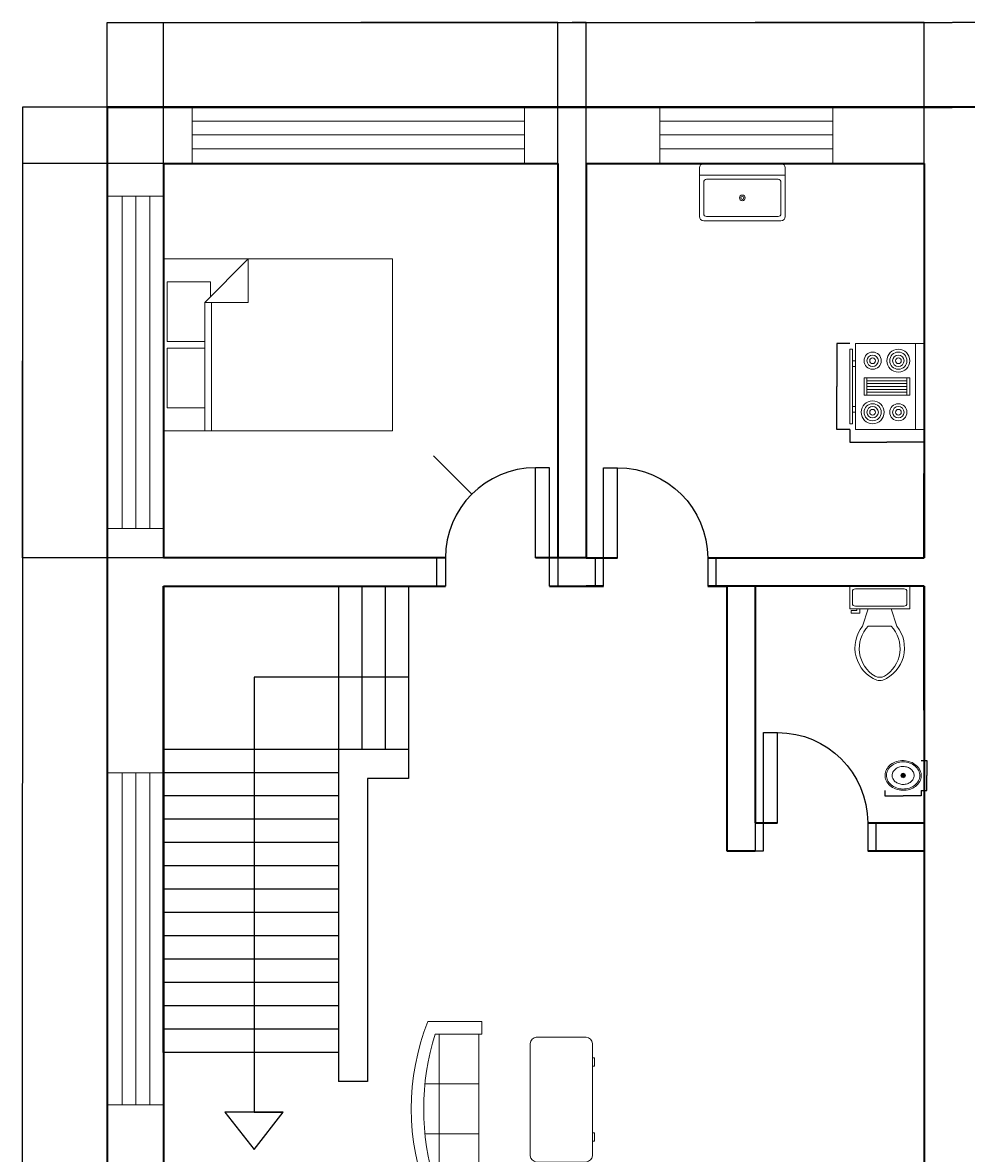
# Model space of a CAD drawing. Units: millimetres. Extents: x 726 to 37095, y -1634 to 13537.
# Tile 1 of 4: x 726 to 9102, y 3500 to 13535. Entities that reach past the tile are written whole.
import ezdxf

# ---------------------------------------------------------------- set-up
doc = ezdxf.new("R2010")
doc.units = ezdxf.units.MM
for name, color, linetype, lineweight in [('A-ANNO-DIMS', 2, 'Continuous', 18), ('A-DOOR', 3, 'Continuous', 25), ('A-EQPM', 8, 'Continuous', 18), ('A-FLOR-FIXT', 9, 'Continuous', 18), ('A-FLOR-STRS', 5, 'Continuous', 25), ('A-FURN', 8, 'Continuous', 18), ('A-GLAZ', 4, 'Continuous', 18), ('A-WALL', 7, 'Continuous', 35)]:
    doc.layers.add(name, color=color, linetype=linetype, lineweight=lineweight)
doc.styles.get("Standard").update_dxf_attribs({"font": 'arial.ttf'})
doc.dimstyles.get("Standard").update_dxf_attribs({"dimtxt": 0.18, "dimasz": 0.18, "dimexe": 0.18, "dimexo": 0.0625, "dimgap": 0.09, "dimtad": 0, "dimtih": 1, "dimtoh": 1, "dimdec": 4, "dimzin": 0, "dimdsep": 46, "dimtxsty": 'Standard', "dimcen": 0.09, "dimadec": 0, "dimazin": 0, "dimtfac": 1, "dimtdec": 4, "dimtofl": 0, "dimtmove": 0, "dimatfit": 3, "dimfxl": 1, "dimtolj": 1, "dimtzin": 0, "dimarcsym": 0})

# ---------------------------------------------------------------- blocks, each defined once
blk = doc.blocks.new('Bed - Queen')
for p, q in [((0, -80.00003000000002), (0, 0)), ((0, 0), (59.99998999999999, 0)), ((59.99998999999999, 0), (59.99998999999999, -80.00003000000002)), ((7.99999, -1.200000000000017), (28.79998, -1.200000000000017)), ((7.99999, -14.4), (7.99999, -1.200000000000017)), ((28.79998, -1.200000000000017), (28.79998, -14.4)), ((31.19999, -1.200000000000017), (51.99999000000001, -1.200000000000017)), ((31.19999, -14.4), (31.19999, -1.200000000000017)), ((51.99999000000001, -1.200000000000017), (51.99999000000001, -16.4)), ((0, -14.4), (44.79999999999999, -14.4)), ((59.99998999999999, -29.60000000000001), (44.79999999999999, -14.4)), ((44.79999999999999, -14.4), (44.79999999999999, -29.60000000000001)), ((44.79999999999999, -16.80000000000001), (0, -16.80000000000001)), ((51.99999000000001, -16.4), (46.79936, -16.4)), ((44.79999999999999, -29.60000000000001), (59.99998999999999, -29.60000000000001)), ((59.99998999999999, -80.00003000000002), (0, -80.00003000000002))]:
    blk.add_line(p, q)
blk = doc.blocks.new('Sofa - Roundback 7 ft.')
for p, q in [((-12.00002, -32.44210000000393), (-12.00003, -6.597100000003898)), ((11.99996999999999, -32.44210000000393), (11.99997999999999, -6.597100000003898)), ((-36.000027, -34.00000000000395), (-36.000027, -11.46960000000396)), ((-35.999844, -13.38190000000397), (35.99979999999999, -13.38190000000397)), ((35.99997999999999, -34.00000000000395), (35.99997999999999, -11.46960000000396)), ((-36.000027, -32.44210000000393), (35.99997999999999, -32.44210000000393))]:
    blk.add_line(p, q)
for points in [[(-36.000027, -34.00000000000395), (-42.000027, -34.00000000000395), (-42.000027, -8.000000000003944)], [(41.99997999999999, -8.000000000003944), (41.99997999999999, -34.00000000000395), (35.99997999999999, -34.00000000000395)]]:
    blk.add_lwpolyline(points)
for centre, radius, start, end in [((0, -114.2500000000039), 114.2500000000039, 68.43141000000072, 111.5686000000006), ((-1.00000000032e-05, -127.1968000000039), 121.1967999999973, 72.72032999999948, 107.2797000000005)]:
    blk.add_arc(centre, radius, start, end)
blk = doc.blocks.new('Desk - 30 x 60 in.')
for p, q in [((-26.999995, 0), (26.999995, 0)), ((-29.999995, -27), (-29.999995, -3)), ((29.999995, -3), (29.999995, -27)), ((26.999995, -30), (-26.999995, -30)), ((-20.000005, -30), (-20.000005, -31)), ((-20.000005, -31), (-16.000005, -31)), ((-16.000005, -31), (-16.000005, -30)), ((15.999995, -31), (15.999995, -30)), ((19.999995, -31), (15.999995, -31)), ((19.999995, -30), (19.999995, -31))]:
    blk.add_line(p, q)
for centre, radius, start, end in [((-26.499995, -3.5), 3.535534000004229, 98.1300999999916, 171.8698999999352), ((26.499995, -3.5), 3.535533999997753, 8.130102000022115, 81.8698999999439), ((-26.499995, -26.5), 3.535534000000845, 188.1301000000653, 261.8699000000085), ((26.499995, -26.5), 3.535534000004826, 278.1301000000561, 351.8698999999439)]:
    blk.add_arc(centre, radius, start, end)
blk = doc.blocks.new('Toilet - top')
for p, q in [((9.5, -6), (9.5, -2)), ((-10, -8.5), (-8, -8.5)), ((-10, -9.5), (-10, -8.5)), ((-7, -9.5), (-10, -9.5)), ((-8, -8.5), (-8, -8)), ((-7, -8), (-7, -9.5)), ((-4, -8), (-6, -14)), ((4, -8), (6, -14)), ((4, -14), (-4, -14))]:
    blk.add_line(p, q)
blk.add_lwpolyline([(10.5, -8), (10.5, 0), (-10.5, 0), (-10.5, -8)], close=True)
for points in [[(-9.5, -2), (-9.5, -6)], [(8.5, -1), (-8.5, -1)], [(-8.5, -7), (8.5, -7)]]:
    blk.add_lwpolyline(points)
for centre, radius, start, end in [((-8.625, -1.875), 0.8838834999999999, 81.86989999999999, 188.1301), ((8.625, -1.875), 0.8838834999999999, 351.8699, 98.13009999999998), ((-8.625, -6.125), 0.8838834999999999, 171.869898, 278.1301), ((8.625, -6.125), 0.8838834999999999, 261.8699, 8.130099999999993), ((3.519562435188956, -21.58049502388982), 12.16902005083646, 141.4691096810948, 247.9714346835576), ((4.199957580658807, -21.81740929088453), 11.3291791325804, 136.3677254423718, 238.946823937405), ((-3.519499936778316, -21.58047137067522), 12.16903423757823, 292.0284332733152, 38.53070636800453), ((-4.199890672038477, -21.81738596564128), 11.32918622148567, 301.0530065773863, 43.63209216694732), ((2.09660981727e-05, -27.87646475467881), 4, 245.7318247449371, 294.2681740488959), ((2.09415214183e-05, -28.99996806116075), 4, 254.8605283244437, 285.1394707718433)]:
    blk.add_arc(centre, radius, start, end)
blk = doc.blocks.new('Sink - Oval top')
for p, q in [((-1, 0), (1, 0)), ((0, 1), (0, -1))]:
    blk.add_line(p, q)
for points in [[(-12.23371880354079, 0.3941914712607968, 0.1176342565883263), (-11.46456229543957, -3.361933235489118, 0.104469279667093), (-8.878748691070427, -6.803541973650567, 0.0900157896014849), (-5.082757700676665, -9.072309807490512, 0.0819199491592185), (-0.3227280122732736, -10.01585280257211, 0.0819199491592091), (4.488169920880977, -9.380701564817912, 0.0900157896014801), (8.422342359155778, -7.36101289847943, 0.1044692796670922), (11.22435122606941, -4.093009071543406, 0.1176342565883338), (12.23371880354091, -0.3941914712607968, 0.1176342565883057), (11.46456229543992, 3.361933235488777, 0.1044692796670849), (8.878748691070427, 6.803541973650567, 0.0900157896014884), (5.082757700676324, 9.072309807490681, 0.0819199491592058), (0.3227280122732736, 10.01585280257211, 0.081919949159207), (-4.488169920880864, 9.380701564817969, 0.0900157896014802), (-8.422342359155778, 7.36101289847943, 0.1044692796670951), (-11.22435122606919, 4.093009071543633, 0.1176342565883402)], [(-11.28627986850119, 0.1590597164737346, 0.1186217001864142), (-10.51590095791209, -3.253161772358112, 0.1046781721811095), (-8.071803350560115, -6.358618019863342, 0.0895620664691738), (-4.537699193222351, -8.366971929609804, 0.0811846988912177), (-0.1289739026695997, -9.15150355811437, 0.0811846988912276), (4.300109150126218, -8.491524865184601, 0.0895620664691798), (7.889406708212618, -6.583562428127606, 0.1046781721811044), (10.42004782883111, -3.548216131892445, 0.1186217001864013), (11.28627986850119, -0.1590597164736209, 0.1186217001863945), (10.51590095791221, 3.253161772357998, 0.1046781721811069), (8.071803350560115, 6.358618019863342, 0.0895620664691756), (4.537699193222124, 8.366971929609917, 0.081184698891216), (0.1289739026695997, 9.151503558114428, 0.0811846988912142), (-4.300109150125877, 8.491524865184829, 0.0895620664691747), (-7.889406708212618, 6.583562428127606, 0.1046781721811045), (-10.42004782883111, 3.548216131892445, 0.1186217001863946)], [(-7.420452389032902, 0.0829876781601797, 0.1182825673856775), (-6.907065465214486, -2.1674649380775, 0.1046074595377274), (-5.294791470712084, -4.209988192029413, 0.0897179636260996), (-2.966599981142508, -5.528122152688069, 0.0814360825277113), (-0.0675135187855176, -6.036810076758797, 0.0814360825277218), (2.84222437824053, -5.593085960977873, 0.0897179636261315), (5.199312936802016, -4.327350491993342, 0.1046074595376878), (6.85686365682659, -2.321395784920355, 0.1182825673856714), (7.420452389033016, -0.0829876781601797, 0.1182825673856961), (6.907065465214486, 2.167464938077614, 0.1046074595377135), (5.294791470712084, 4.209988192029413, 0.0897179636261265), (2.966599981142621, 5.528122152687842, 0.0814360825277426), (0.0675135187855176, 6.036810076758797, 0.0814360825277225), (-2.842224378240644, 5.593085960977873, 0.0897179636261212), (-5.199312936802016, 4.327350491993342, 0.1046074595377049), (-6.856863656826476, 2.321395784920355, 0.1182825673856712)]]:
    blk.add_lwpolyline(points, format="xyb", close=True)
for radius in [1.5, 1]:
    blk.add_circle((0, 0), radius)
blk = doc.blocks.new('Range-Oven - 30 in top')
for p, q in [((0, -3), (30, -3)), ((12, -6), (18, -6)), ((13, -19.999996), (13, -6)), ((14, -6), (14, -19.999996)), ((15, -19.999996), (15, -6)), ((16, -6), (16, -19.999996)), ((17, -19.999996), (17, -6)), ((18, -19.999996), (12, -19.999996)), ((6.000000000000003, -23.99999600000001), (6.000000000000003, -24.999996)), ((8.000000000000004, -24.999996), (8.000000000000004, -23.99999600000001)), ((22.00000000000001, -24.999996), (22.00000000000001, -23.99999600000001)), ((24, -23.99999600000001), (24, -24.999996))]:
    blk.add_line(p, q)
for points in [[(0, -23.99999600000001), (0, 0), (30, 0), (30, -23.99999600000001)], [(12, -20.999996), (12, -5), (18, -5), (18, -20.999996)], [(2.000000000000003, -25.999996), (2.000000000000003, -24.999996), (28.00000000000001, -24.999996), (28.00000000000001, -25.999996)]]:
    blk.add_lwpolyline(points, close=True)
for centre, radius in [((6.000000000000003, -9.0000002), 4), ((6.000000000000003, -9.0000002), 3), ((6.000000000000003, -9.0000002), 2), ((24, -9.0000002), 3), ((24, -9.0000002), 2), ((6.000000000000003, -9.0000002), 1), ((24, -9.0000002), 1), ((6.000000000000003, -18), 3), ((24, -18), 4), ((24, -18), 3), ((6.000000000000003, -18), 2), ((6.000000000000003, -18), 1), ((24, -18), 2), ((24, -18), 1)]:
    blk.add_circle(centre, radius)
blk = doc.blocks.new('Sink-single - 30 in top')
blk.add_line((-15, -3.999996000000001), (15, -3.999996000000001))
for points in [[(-13.5, 0), (13.5, 0)], [(-15, -18.499996), (-15, -1.500000000000001)], [(15, -1.500000000000001), (15, -18.499996)], [(-13.5, -17.499996), (-13.5, -6.499996000000001)], [(-12.5, -5.499996000000001), (12.5, -5.499996000000001)], [(13.5, -6.499996000000001), (13.5, -17.499996)], [(12.5, -18.499996), (-12.5, -18.499996)], [(13.5, -19.999996), (-13.5, -19.999996)]]:
    blk.add_lwpolyline(points)
for radius in [1, 0.5]:
    blk.add_circle((0, -11.999996), radius)
for centre, radius, start, end in [((-13.5, -1.500000000000001), 1.5, 90, 180), ((13.5, -1.500000000000001), 1.5, 0, 90), ((-12.5, -6.499996000000001), 1, 90, 180), ((12.5, -6.499996000000001), 1, 0, 90), ((-13.5, -18.499996), 1.5, 180, 270), ((-12.5, -17.499996), 1, 180, 270), ((12.5, -17.499996), 1, 270, 0), ((13.5, -18.499996), 1.5, 270, 0)]:
    blk.add_arc(centre, radius, start, end)
blk = doc.blocks.new('Window - Wood Frame 36 in. Wide plan')
for p, q in [((0, 6), (0, 0)), ((36, 6), (36, 0)), ((0, 4.5), (36, 4.5)), ((0, 3), (36, 3)), ((0, 1.5), (36, 1.5))]:
    blk.add_line(p, q)
blk = doc.blocks.new('DOOR-SWING-800')
for p, q in [((999.1999999999979, 1050), (874.1999999999979, 1050)), ((874.1999999999979, 250), (874.1999999999979, 1050)), ((999.1999999999979, 250), (999.1999999999979, 1050)), ((9.095e-13, 250), (74.199999999998, 250)), ((9.095e-13, 0), (9.095e-13, 250)), ((74.199999999998, 250), (74.199999999998, 0)), ((874.1999999999979, 250), (999.1999999999979, 250)), ((999.1999999999979, 250), (1073.400000000002, 250)), ((999.1999999999979, 0), (999.1999999999979, 250)), ((1073.400000000002, 250), (1073.400000000002, 0)), ((74.199999999998, 0), (9.095e-13, 0)), ((1073.400000000002, 0), (999.1999999999979, 0))]:
    blk.add_line(p, q)
blk.add_arc((874.1999999999979, 250), 800, 90, 180)
blk = doc.blocks.new('STAIR-QUARTER-TURN')
for p, q in [((1551.94660387568, 5000.000000000002), (1551.94660387568, 3551.516503049365)), ((1758.872817725773, 5000.000000000002), (1758.872817725773, 3551.516503049365)), ((1965.799031575862, 5000.000000000002), (1965.799031575862, 3551.516503049365)), ((2172.725245425954, 5000.000000000002), (2172.725245425954, 3551.516503049365)), ((2172.725245425954, 4193.579423830473), (803.743340616409, 4193.579423830471)), ((803.743340616409, 4193.579423830471), (803.743340616409, 330.5564002077117)), ((2172.725245425954, 3551.516503049366), (0, 3551.516503049365)), ((1551.94660387568, 3551.516503049365), (1551.94660387568, 3344.590289199272)), ((2172.725245425954, 3551.516503049365), (2172.725245425954, 3292.858735736751)), ((1551.94660387568, 3344.590289199272), (0, 3344.590289199273)), ((1551.94660387568, 3344.590289199272), (1551.94660387568, 861.4757229981805)), ((2172.725245425954, 3292.858735736751), (1810.604371188295, 3292.858735736751)), ((1810.604371188295, 3292.85873573675), (1810.604371188295, 602.8179556856148)), ((1551.94660387568, 3137.664075349182), (0, 3137.664075349182)), ((1551.94660387568, 2930.73786149909), (0, 2930.737861499091)), ((1551.94660387568, 2723.811647649), (0, 2723.811647649001)), ((1551.94660387568, 2516.885433798908), (0, 2516.885433798909)), ((1551.94660387568, 2309.959219948817), (0, 2309.959219948818)), ((1551.94660387568, 2103.033006098726), (0, 2103.033006098727)), ((1551.94660387568, 1896.106792248635), (0, 1896.106792248635)), ((1551.94660387568, 1689.180578398543), (0, 1689.180578398544)), ((1551.94660387568, 1482.254364548453), (0, 1482.254364548454)), ((1551.94660387568, 1275.328150698362), (0, 1275.328150698363)), ((1551.94660387568, 1068.40193684827), (0, 1068.401936848271)), ((1551.94660387568, 861.4757229981795), (0, 861.4757229981805)), ((1551.94660387568, 861.4757229981805), (1551.946603875687, 602.8179556856074)), ((1810.604371188295, 602.8179556856148), (1551.946603875687, 602.8179556855675)), ((803.743340616409, 330.5564002077117), (545.0855733037969, 330.5564002077117)), ((545.0855733037969, 330.5564002077117), (803.743340616409, 4.547e-13)), ((803.743340616409, 330.5564002077117), (1062.401107929021, 330.5564002077108)), ((803.743340616409, 4.547e-13), (1062.401107929021, 330.5564002077117))]:
    blk.add_line(p, q)
blk = doc.blocks.new('WIN-1535')
for p, q in [((0, 1.819e-12), (0, 500.0000000000036)), ((1534.861597237876, 1.819e-12), (1534.861597237876, 500.0000000000036)), ((-9.095e-13, 377.1532172399693), (1534.861597237876, 377.1532172399693)), ((-9.095e-13, 254.306434479935), (1534.861597237876, 254.306434479935)), ((-9.095e-13, 131.459651719897), (1534.861597237876, 131.4596517198988))]:
    blk.add_line(p, q)
blk = doc.blocks.new('*D33')
at = {"layer": 'A-ANNO-DIMS', "color": 0, "lineweight": -2, "transparency": 16777216}
for p, q in [((8379.49967440098, 6721.430037603937), (8379.49967440098, 6672.895314363273)), ((8379.67967440098, 6673.075314363273), (8539.884149777998, 6673.075314363273)), ((8702.10116267207, 6673.075314363273), (8541.896687295051, 6673.075314363273)), ((8702.28116267207, 6721.430037603937), (8702.28116267207, 6672.895314363273))]:
    blk.add_line(p, q, dxfattribs=at)
at = {"layer": 'A-ANNO-DIMS', "color": 0, "transparency": 16777216}
for points in [[(8379.67967440098, 6673.105314363273), (8379.67967440098, 6673.045314363275), (8379.49967440098, 6673.075314363273)], [(8702.10116267207, 6673.105314363273), (8702.10116267207, 6673.045314363275), (8702.28116267207, 6673.075314363273)]]:
    blk.add_solid(points, dxfattribs=at)
at = {"layer": 'Defpoints', "color": 0, "transparency": 16777216}
for p in [(8379.49967440098, 6721.492537603937), (8702.28116267207, 6721.492537603937), (8702.28116267207, 6673.075314363273)]:
    blk.add_point(p, dxfattribs=at)
at = {"layer": 'A-ANNO-DIMS', "color": 0, "transparency": 16777216, "insert": (8540.890418536525, 6673.075314363273), "char_height": 0.18, "attachment_point": 5}
blk.add_mtext('\\A1;BASIN 323 TYP.', dxfattribs=at)
blk = doc.blocks.new('*D34')
at = {"layer": 'A-ANNO-DIMS', "color": 0, "lineweight": -2, "transparency": 16777216}
for p, q in [((8702.343662672074, 6986.237226650004), (8750.878385912742, 6986.237226650004)), ((8750.698385912741, 6986.057226650004), (8750.698385912741, 6854.046785264762)), ((8750.698385912741, 6721.672537603942), (8750.698385912741, 6853.682978989183)), ((8702.343662672074, 6721.492537603942), (8750.878385912742, 6721.492537603942))]:
    blk.add_line(p, q, dxfattribs=at)
at = {"layer": 'A-ANNO-DIMS', "color": 0, "transparency": 16777216}
for points in [[(8750.66838591274, 6986.057226650004), (8750.728385912742, 6986.057226650004), (8750.698385912741, 6986.237226650004)], [(8750.66838591274, 6721.672537603942), (8750.728385912742, 6721.672537603942), (8750.698385912741, 6721.492537603942)]]:
    blk.add_solid(points, dxfattribs=at)
at = {"layer": 'Defpoints', "color": 0, "transparency": 16777216}
for p in [(8702.281162672074, 6986.237226650004), (8750.698385912741, 6986.237226650004), (8702.281162672074, 6721.492537603942)]:
    blk.add_point(p, dxfattribs=at)
at = {"layer": 'A-ANNO-DIMS', "color": 0, "transparency": 16777216, "insert": (8750.698385912741, 6853.864882126969), "char_height": 0.18, "attachment_point": 5}
blk.add_mtext('\\A1;265 TYP.', dxfattribs=at)
blk = doc.blocks.new('*D37')
at = {"layer": 'A-ANNO-DIMS', "color": 0, "lineweight": -2, "transparency": 16777216}
for p, q in [((8066.847447465294, 10686.62375609469), (7952.429947465296, 10686.62375609469)), ((7952.609947465297, 10686.44375609469), (7952.609947465297, 10305.80682567177)), ((7952.609947465298, 9924.803756094694), (7952.609947465297, 10305.44068651761)), ((8066.847447465294, 9924.623756094694), (7952.429947465297, 9924.623756094694))]:
    blk.add_line(p, q, dxfattribs=at)
at = {"layer": 'A-ANNO-DIMS', "color": 0, "transparency": 16777216}
for points in [[(7952.579947465297, 10686.44375609469), (7952.639947465296, 10686.44375609469), (7952.609947465297, 10686.62375609469)], [(7952.579947465299, 9924.803756094694), (7952.639947465297, 9924.803756094694), (7952.609947465298, 9924.623756094694)]]:
    blk.add_solid(points, dxfattribs=at)
at = {"layer": 'Defpoints', "color": 0, "transparency": 16777216}
for p in [(8066.909947465294, 10686.62375609469), (7952.609947465298, 9924.623756094694), (8066.909947465294, 9924.623756094694)]:
    blk.add_point(p, dxfattribs=at)
at = {"layer": 'A-ANNO-DIMS', "color": 0, "transparency": 16777216, "insert": (7952.609947465298, 10305.62375609469), "char_height": 0.18, "attachment_point": 5}
blk.add_mtext('\\A1;RANGE 762 TYP.', dxfattribs=at)
blk = doc.blocks.new('*D38')
at = {"layer": 'A-ANNO-DIMS', "color": 0, "lineweight": -2, "transparency": 16777216}
for p, q in [((8066.909947465289, 9924.56125609469), (8066.909947465289, 9810.14375609469)), ((8727.30984586529, 9924.56125609469), (8727.30984586529, 9810.14375609469)), ((8067.089947465289, 9810.32375609469), (8396.511390526133, 9810.32375609469)), ((8727.12984586529, 9810.32375609469), (8397.708402804445, 9810.32375609469))]:
    blk.add_line(p, q, dxfattribs=at)
at = {"layer": 'A-ANNO-DIMS', "color": 0, "transparency": 16777216}
for points in [[(8067.089947465289, 9810.353756094692), (8067.089947465289, 9810.29375609469), (8066.909947465289, 9810.32375609469)], [(8727.12984586529, 9810.353756094692), (8727.12984586529, 9810.29375609469), (8727.30984586529, 9810.32375609469)]]:
    blk.add_solid(points, dxfattribs=at)
at = {"layer": 'Defpoints', "color": 0, "transparency": 16777216}
for p in [(8066.909947465289, 9924.62375609469), (8727.30984586529, 9924.62375609469), (8727.30984586529, 9810.32375609469)]:
    blk.add_point(p, dxfattribs=at)
at = {"layer": 'A-ANNO-DIMS', "color": 0, "transparency": 16777216, "insert": (8397.10989666529, 9810.32375609469), "char_height": 0.18, "attachment_point": 5}
blk.add_mtext('\\A1;660 TYP.', dxfattribs=at)
blk = doc.blocks.new('*D43')
at = {"layer": 'A-ANNO-DIMS', "color": 0, "lineweight": -2, "transparency": 16777216}
for p, q in [((1477.309846, 12783.948368), (1477.309846, 13534.815868)), ((1477.489846, 13534.635868), (8976.889927855387, 13534.635868)), ((16477.129846, 13534.635868), (8977.72976414461, 13534.635868)), ((16477.309846, 12783.948368), (16477.309846, 13534.815868))]:
    blk.add_line(p, q, dxfattribs=at)
at = {"layer": 'A-ANNO-DIMS', "color": 0, "transparency": 16777216}
for points in [[(1477.489846, 13534.665868), (1477.489846, 13534.605868), (1477.309846, 13534.635868)], [(16477.129846, 13534.665868), (16477.129846, 13534.605868), (16477.309846, 13534.635868)]]:
    blk.add_solid(points, dxfattribs=at)
at = {"layer": 'Defpoints', "color": 0, "transparency": 16777216}
for p in [(16477.309846, 13534.635868), (1477.309846, 12783.885868), (16477.309846, 12783.885868)]:
    blk.add_point(p, dxfattribs=at)
at = {"layer": 'A-ANNO-DIMS', "color": 0, "transparency": 16777216, "insert": (8977.309846, 13534.635868), "char_height": 0.18, "attachment_point": 5}
blk.add_mtext('\\A1;15000', dxfattribs=at)
blk = doc.blocks.new('*D44')
at = {"layer": 'A-ANNO-DIMS', "color": 0, "lineweight": -2, "transparency": 16777216}
for p, q in [((1477.247346, 12783.885868), (726.3798459999991, 12783.885868)), ((726.559845999999, 12783.705868), (726.5598460000004, 6784.067771137793)), ((726.5598460000017, 784.0658680000001), (726.5598460000004, 6783.703964862214)), ((1477.247346, 783.8858680000003), (726.3798460000017, 783.8858680000002))]:
    blk.add_line(p, q, dxfattribs=at)
at = {"layer": 'A-ANNO-DIMS', "color": 0, "transparency": 16777216}
for points in [[(726.5298459999991, 12783.705868), (726.589845999999, 12783.705868), (726.559845999999, 12783.885868)], [(726.5298460000017, 784.0658680000001), (726.5898460000016, 784.0658680000001), (726.5598460000017, 783.8858680000002)]]:
    blk.add_solid(points, dxfattribs=at)
at = {"layer": 'Defpoints', "color": 0, "transparency": 16777216}
for p in [(726.559845999999, 12783.885868), (1477.309846, 12783.885868), (1477.309846, 783.8858680000003)]:
    blk.add_point(p, dxfattribs=at)
at = {"layer": 'A-ANNO-DIMS', "color": 0, "transparency": 16777216, "insert": (726.5598460000022, 6783.885868000002), "char_height": 0.18, "attachment_point": 5}
blk.add_mtext('\\A1;12000', dxfattribs=at)
blk = doc.blocks.new('*D45')
at = {"layer": 'A-ANNO-DIMS', "color": 0, "lineweight": -2, "transparency": 16777216}
for p, q in [((1977.309846, 12283.948368), (1977.309846, 13534.815868)), ((1977.489846, 13534.635868), (3726.951442180082, 13534.635868)), ((5477.129846, 13534.635868), (3727.668249819919, 13534.635868)), ((5477.309846, 12283.948368), (5477.309846, 13534.815868))]:
    blk.add_line(p, q, dxfattribs=at)
at = {"layer": 'A-ANNO-DIMS', "color": 0, "transparency": 16777216}
for points in [[(1977.489846, 13534.665868), (1977.489846, 13534.605868), (1977.309846, 13534.635868)], [(5477.129846, 13534.665868), (5477.129846, 13534.605868), (5477.309846, 13534.635868)]]:
    blk.add_solid(points, dxfattribs=at)
at = {"layer": 'Defpoints', "color": 0, "transparency": 16777216}
for p in [(5477.309846, 13534.635868), (1977.309846, 12283.885868), (5477.309846, 12283.885868)]:
    blk.add_point(p, dxfattribs=at)
at = {"layer": 'A-ANNO-DIMS', "color": 0, "transparency": 16777216, "insert": (3727.309846, 13534.635868), "char_height": 0.18, "attachment_point": 5}
blk.add_mtext('\\A1;3500', dxfattribs=at)
blk = doc.blocks.new('*D46')
at = {"layer": 'A-ANNO-DIMS', "color": 0, "lineweight": -2, "transparency": 16777216}
for p, q in [((5477.309846, 12283.948368), (5477.309846, 13534.815868)), ((5477.489846, 13534.635868), (5602.019770965893, 13534.635868)), ((5727.129846, 13534.635868), (5602.599921034107, 13534.635868)), ((5727.309846, 12283.948368), (5727.309846, 13534.815868))]:
    blk.add_line(p, q, dxfattribs=at)
at = {"layer": 'A-ANNO-DIMS', "color": 0, "transparency": 16777216}
for points in [[(5477.489846, 13534.665868), (5477.489846, 13534.605868), (5477.309846, 13534.635868)], [(5727.129846, 13534.665868), (5727.129846, 13534.605868), (5727.309846, 13534.635868)]]:
    blk.add_solid(points, dxfattribs=at)
at = {"layer": 'Defpoints', "color": 0, "transparency": 16777216}
for p in [(5727.309846, 13534.635868), (5477.309846, 12283.885868), (5727.309846, 12283.885868)]:
    blk.add_point(p, dxfattribs=at)
at = {"layer": 'A-ANNO-DIMS', "color": 0, "transparency": 16777216, "insert": (5602.309846, 13534.635868), "char_height": 0.18, "attachment_point": 5}
blk.add_mtext('\\A1;250', dxfattribs=at)
blk = doc.blocks.new('*D47')
at = {"layer": 'A-ANNO-DIMS', "color": 0, "lineweight": -2, "transparency": 16777216}
for p, q in [((5727.309846, 12283.948368), (5727.309846, 13534.815868)), ((5727.489846, 13534.635868), (7226.951442180082, 13534.635868)), ((8727.129846, 13534.635868), (7227.668249819918, 13534.635868)), ((8727.309846, 12283.948368), (8727.309846, 13534.815868))]:
    blk.add_line(p, q, dxfattribs=at)
at = {"layer": 'A-ANNO-DIMS', "color": 0, "transparency": 16777216}
for points in [[(5727.489846, 13534.665868), (5727.489846, 13534.605868), (5727.309846, 13534.635868)], [(8727.129846, 13534.665868), (8727.129846, 13534.605868), (8727.309846, 13534.635868)]]:
    blk.add_solid(points, dxfattribs=at)
at = {"layer": 'Defpoints', "color": 0, "transparency": 16777216}
for p in [(8727.309846, 13534.635868), (5727.309846, 12283.885868), (8727.309846, 12283.885868)]:
    blk.add_point(p, dxfattribs=at)
at = {"layer": 'A-ANNO-DIMS', "color": 0, "transparency": 16777216, "insert": (7227.309846, 13534.635868), "char_height": 0.18, "attachment_point": 5}
blk.add_mtext('\\A1;3000', dxfattribs=at)
blk = doc.blocks.new('*D48')
at = {"layer": 'A-ANNO-DIMS', "color": 0, "lineweight": -2, "transparency": 16777216}
for p, q in [((8727.309846, 12283.948368), (8727.309846, 13534.815868)), ((8727.489846, 13534.635868), (8977.021305754433, 13534.635868)), ((9227.129846, 13534.635868), (8977.598386245567, 13534.635868)), ((9227.309846, 12283.948368), (9227.309846, 13534.815868))]:
    blk.add_line(p, q, dxfattribs=at)
at = {"layer": 'A-ANNO-DIMS', "color": 0, "transparency": 16777216}
for points in [[(8727.489846, 13534.665868), (8727.489846, 13534.605868), (8727.309846, 13534.635868)], [(9227.129846, 13534.665868), (9227.129846, 13534.605868), (9227.309846, 13534.635868)]]:
    blk.add_solid(points, dxfattribs=at)
at = {"layer": 'Defpoints', "color": 0, "transparency": 16777216}
for p in [(9227.309846, 13534.635868), (8727.309846, 12283.885868), (9227.309846, 12283.885868)]:
    blk.add_point(p, dxfattribs=at)
at = {"layer": 'A-ANNO-DIMS', "color": 0, "transparency": 16777216, "insert": (8977.309846, 13534.635868), "char_height": 0.18, "attachment_point": 5}
blk.add_mtext('\\A1;500', dxfattribs=at)
blk = doc.blocks.new('*D53')
at = {"layer": 'A-ANNO-DIMS', "color": 0, "lineweight": -2, "transparency": 16777216}
for p, q in [((1977.247346000001, 12283.885868), (726.3798460000002, 12283.885868)), ((726.5598460000001, 12283.705868), (726.5598460000004, 10534.06783252933)), ((726.5598460000009, 8784.065868000003), (726.5598460000004, 10533.70390347067)), ((1977.247346000001, 8783.885868000005), (726.3798460000007, 8783.885868000005))]:
    blk.add_line(p, q, dxfattribs=at)
at = {"layer": 'A-ANNO-DIMS', "color": 0, "transparency": 16777216}
for points in [[(726.5298460000001, 12283.705868), (726.589846, 12283.705868), (726.5598460000001, 12283.885868)], [(726.5298460000009, 8784.065868000003), (726.5898460000008, 8784.065868000003), (726.5598460000009, 8783.885868000005)]]:
    blk.add_solid(points, dxfattribs=at)
at = {"layer": 'Defpoints', "color": 0, "transparency": 16777216}
for p in [(1977.309846000001, 12283.885868), (726.5598460000009, 8783.885868000005), (1977.309846000001, 8783.885868000005)]:
    blk.add_point(p, dxfattribs=at)
at = {"layer": 'A-ANNO-DIMS', "color": 0, "transparency": 16777216, "insert": (726.5598460000034, 10533.885868), "char_height": 0.18, "attachment_point": 5}
blk.add_mtext('\\A1;3500', dxfattribs=at)
blk = doc.blocks.new('*D85')
at = {"layer": 'A-ANNO-DIMS', "color": 0, "lineweight": -2, "transparency": 16777216}
for p, q in [((4372.832594830522, 9688.981976769475), (4373.012594830522, 9688.981976769475)), ((4373.012594830522, 9688.981976769475), (4712.29678469906, 9349.69821514029)), ((5278.019845999999, 8783.885867999996), (5278.199846, 8783.885868)), ((5278.109846, 8783.795868), (5278.109846, 8783.975868))]:
    blk.add_line(p, q, dxfattribs=at)
at = {"layer": 'A-ANNO-DIMS', "color": 0, "transparency": 16777216}
blk.add_solid([(4712.317997889108, 9349.719428357112), (4712.275571509011, 9349.677001923465), (4712.424063999999, 9349.570936)], dxfattribs=at)
at = {"layer": 'Defpoints', "color": 0, "transparency": 16777216}
for p in [(4712.424063999999, 9349.570936), (5278.109845999999, 8783.885868)]:
    blk.add_point(p, dxfattribs=at)
at = {"layer": 'A-ANNO-DIMS', "color": 0, "transparency": 16777216, "insert": (4372.264047763674, 9688.981976769477), "char_height": 0.18, "attachment_point": 5}
blk.add_mtext('\\A1;6X R800', dxfattribs=at)

msp = doc.modelspace()

# ---------------------------------------------------------------- linework, layer by layer
at = {"layer": 'A-DOOR'}
for p, q in [((5403.109845865284, 8783.885868122885), (5278.109845865284, 8783.885868122885)), ((5807.038045798428, 8783.885868122887), (5807.038045798428, 8533.885868122887)), ((5881.238045798433, 8783.885868122887), (6006.238045798433, 8783.885868122887)), ((7227.309845865285, 6434.561644066505), (7227.309845865285, 6184.561644066505)), ((7301.50984586529, 6434.561644066505), (7426.50984586529, 6434.561644066505)), ((7227.309845865287, 6184.561644066505), (7301.50984586529, 6184.561644066505))]:
    msp.add_line(p, q, dxfattribs=at)
at = {"layer": 'A-FLOR-STRS'}
for p, q in [((2781.053186481699, 7727.465291953355), (2781.053186481699, 7727.465291953355)), ((3039.710953794312, 3864.442268330595), (2781.053186481699, 3864.442268330595))]:
    msp.add_line(p, q, dxfattribs=at)
at = {"layer": 'A-WALL'}
for p, q in [((16477.30984586529, 12783.88586812288), (1477.309845865288, 12783.88586812288)), ((1477.309845865288, 12783.88586812288), (1477.309845865288, 783.8858681228857)), ((1477.309845865288, 12783.88586812288), (8977.309845865288, 12783.88586812288)), ((1477.309845865288, 12783.88586812288), (4977.309845865288, 12783.88586812288)), ((1477.309845865288, 12783.88586812288), (1977.309845865287, 12783.88586812288)), ((1477.309845865288, 12783.88586812288), (1477.309845865288, 12783.88586812288)), ((1477.309845865288, 12783.88586812288), (1477.309845865288, 12283.88586812288)), ((8977.309845865288, 12783.88586812288), (5977.309845865288, 12783.88586812288)), ((1977.309845865287, 12283.88586812288), (1977.309845865287, 8783.885868122885)), ((1977.309845865287, 12283.88586812288), (5477.309845865288, 12283.88586812288)), ((5477.309845865288, 12283.88586812288), (5477.309845865288, 8783.885868122885)), ((5727.309845865288, 12283.88586812288), (5727.309845865288, 9283.885868122885)), ((5727.309845865288, 12283.88586812288), (8727.30984586529, 12283.88586812288)), ((8727.30984586529, 12283.88586812288), (8727.30984586529, 8784.561644066505)), ((8727.309845865288, 9783.885868122887), (8727.309845865288, 9533.885868122885)), ((8727.309845865288, 8784.561644066505), (8727.309845865288, 9533.885868122885)), ((1977.309845865287, 9283.885868122885), (1977.309845865287, 9033.885868122885)), ((5727.309845865288, 9283.885868122885), (5727.309845865288, 9033.885868122885)), ((5727.309845865288, 9033.885868122885), (5727.309845865288, 8783.885868122885)), ((4478.109845865283, 8783.885868122885), (1977.309845865287, 8783.885868122885)), ((5477.309845865288, 8783.885868122885), (5278.109845865284, 8783.885868122885)), ((5727.309845865288, 8783.885868122885), (5477.309845865288, 8783.885868122885)), ((5727.309845865288, 8784.561644066505), (6006.238045798433, 8784.561644066505)), ((6806.237760377678, 8784.561644066505), (8727.309845865288, 8784.561644066505)), ((1977.309845865287, 8533.885868122885), (4478.109845865283, 8533.885868122887)), ((1977.309845865287, 4395.361591121064), (1977.309845865287, 8533.885868122885)), ((1977.309845865287, 8533.885868122885), (4478.109845865283, 8533.885868122885)), ((1977.309845865287, 8533.885868122883), (1977.309845865287, 1283.885868122886)), ((5403.109845865284, 8533.885868122887), (5881.238045798433, 8533.885868122887)), ((5881.238045798433, 8534.561644066505), (5727.309845865288, 8534.561644066505)), ((8727.309845865288, 8534.561644066505), (6806.238045798433, 8534.561644066505)), ((6806.238045798433, 8533.885868122887), (6977.309845865288, 8533.885868122887)), ((6977.309845865288, 8534.561644066505), (6977.309845865288, 6434.561644066507)), ((7227.309845865288, 8534.561644066505), (7227.309845865288, 6434.561644066505)), ((8727.309845865288, 7433.885868122882), (8727.309845865288, 8534.561644066505)), ((8727.30984586529, 8534.561644066505), (8727.309845865288, 1283.885868122885)), ((6977.309845865288, 6434.561644066507), (6977.309845865287, 6184.561644066505)), ((7227.309845865288, 6434.561644066505), (7426.50984586529, 6434.561644066505)), ((8226.50984586529, 6434.561644066505), (8727.309845865288, 6434.561644066505)), ((6977.309845865287, 6184.561644066505), (7227.309845865287, 6184.561644066505)), ((8226.509845865288, 6184.561644066505), (8727.30984586529, 6184.561644066505))]:
    msp.add_line(p, q, dxfattribs=at)

# ---------------------------------------------------------------- block references
at = {"layer": 'A-DOOR'}
msp.add_blockref('DOOR-SWING-800', (4403.909845865284, 8533.885868122885), dxfattribs=at)
at = {"layer": 'A-DOOR', "extrusion": (0, 0, -1), "zscale": -1}
for p in [(-6880.438045798434, 8533.885868122885), (-8300.709845865284, 6184.5616440665)]:
    msp.add_blockref('DOOR-SWING-800', p, dxfattribs=at)
at = {"layer": 'A-EQPM', "xscale": 25.4, "yscale": 25.4, "zscale": 25.4, "rotation": 270}
msp.add_blockref('Range-Oven - 30 in top', (8727.30984586529, 10686.62375609469), dxfattribs=at)
at = {"layer": 'A-FLOR-FIXT'}
for name, p, xscale, yscale, zscale in [('Sink-single - 30 in top', (7113.817916848166, 12283.88586812288), 25.4, 25.4, 25.4), ('Toilet - top', (8333.198180601526, 8534.561644066505), 25.4, 25.4, 25.4), ('Sink - Oval top', (8540.890418536525, 6853.864882126969), 13.14744327818227, 13.14744327818227, 13.14744327818227)]:
    msp.add_blockref(name, p, dxfattribs=dict(at, xscale=xscale, yscale=yscale, zscale=zscale))
at = {"layer": 'A-FLOR-STRS'}
msp.add_blockref('STAIR-QUARTER-TURN', (1977.309845865304, 3533.885868122879), dxfattribs=at)
at = {"layer": 'A-FURN', "rotation": 90}
for name, p, xscale, yscale, zscale in [('Bed - Queen', (1977.309845865287, 9913.47188921653), 25.4, 25.4, 25.4), ('Sofa - Roundback 7 ft.', (4175.152231439681, 3894.653569822566), 18.46049527356076, 18.46049527356076, 18.46049527356076), ('Desk - 30 x 60 in.', (5229.86281300102, 3977.274990980613), 18.46049527356076, 18.46049527356076, 18.46049527356076)]:
    msp.add_blockref(name, p, dxfattribs=dict(at, xscale=xscale, yscale=yscale, zscale=zscale))
at = {"layer": 'A-GLAZ', "xscale": 81.8978551733564, "yscale": 81.8978551733564, "zscale": 81.8978551733564}
msp.add_blockref('Window - Wood Frame 36 in. Wide plan', (2231.692889473896, 12292.49873708274), dxfattribs=at)
at = {"layer": 'A-GLAZ'}
msp.add_blockref('WIN-1535', (6382.166362054324, 12283.88586812288), dxfattribs=at)
at = {"layer": 'A-GLAZ', "xscale": 81.8978551733564, "yscale": 81.8978551733564, "zscale": 81.8978551733564, "rotation": 270}
for p in [(1485.922714825149, 11993.94509580379), (1485.922714825149, 6878.476157322156)]:
    msp.add_blockref('Window - Wood Frame 36 in. Wide plan', p, dxfattribs=at)

# ---------------------------------------------------------------- dimensions: what is measured, and where the dimension line sits
at = {"layer": 'A-ANNO-DIMS'}
for base, p1, p2, picture, middle in [((16477.309846, 13534.635868), (1477.309846, 12783.885868), (16477.309846, 12783.885868), '*D43', (8977.309846, 13534.635868)), ((5477.309846, 13534.635868), (1977.309846, 12283.885868), (5477.309846, 12283.885868), '*D45', (3727.309846, 13534.635868)), ((5727.309846, 13534.635868), (5477.309846, 12283.885868), (5727.309846, 12283.885868), '*D46', (5602.309846, 13534.635868)), ((8727.309846, 13534.635868), (5727.309846, 12283.885868), (8727.309846, 12283.885868), '*D47', (7227.309846, 13534.635868)), ((9227.309846, 13534.635868), (8727.309846, 12283.885868), (9227.309846, 12283.885868), '*D48', (8977.309846, 13534.635868))]:
    dim = msp.add_linear_dim(base=base, p1=p1, p2=p2, dimstyle='Standard', override={"dimdec": 0, "dimlfac": 1, "dimrnd": 0, "dimzin": 0, "dimdsep": 46, "dimlunit": 2}, dxfattribs=at)
    dim.commit()
    dim.dimension.update_dxf_attribs({"geometry": picture, "text_midpoint": middle})
for base, p1, p2, picture, middle in [((726.559845999999, 12783.885868), (1477.309846, 783.8858679999998), (1477.309846, 12783.885868), '*D44', (726.5598460000022, 6783.885868000002)), ((726.5598460000009, 8783.885868000005), (1977.309846, 12283.885868), (1977.309846, 8783.885868), '*D53', (726.5598460000034, 10533.885868))]:
    dim = msp.add_linear_dim(base=base, p1=p1, p2=p2, angle=90, dimstyle='Standard', override={"dimdec": 0, "dimlfac": 1, "dimrnd": 0, "dimzin": 0, "dimdsep": 46, "dimlunit": 2}, dxfattribs=at)
    dim.commit()
    dim.dimension.update_dxf_attribs({"geometry": picture, "text_midpoint": middle})
for base, p1, p2, angle, text, picture, middle in [((7952.609947465298, 9924.623756094694), (8066.909947465289, 10686.62375609469), (8066.909947465289, 9924.62375609469), 270, 'RANGE <> TYP.', '*D37', (7952.609947465298, 10305.62375609469)), ((8750.698385912741, 6986.237226650004), (8702.28116267207, 6721.492537603937), (8702.28116267207, 6986.237226650001), 90, '<> TYP.', '*D34', (8750.698385912741, 6853.864882126969))]:
    dim = msp.add_linear_dim(base=base, p1=p1, p2=p2, angle=angle, text=text, dimstyle='Standard', override={"dimdec": 0, "dimlfac": 1, "dimrnd": 0, "dimzin": 0, "dimdsep": 46, "dimlunit": 2}, dxfattribs=at)
    dim.commit()
    dim.dimension.update_dxf_attribs({"geometry": picture, "text_midpoint": middle})
for base, p1, p2, text, picture, middle in [((8727.30984586529, 9810.32375609469), (8066.909947465289, 9924.62375609469), (8727.30984586529, 9924.62375609469), '<> TYP.', '*D38', (8397.10989666529, 9810.32375609469)), ((8702.28116267207, 6673.075314363273), (8379.49967440098, 6721.492537603937), (8702.28116267207, 6721.492537603937), 'BASIN <> TYP.', '*D33', (8540.890418536525, 6673.075314363273))]:
    dim = msp.add_linear_dim(base=base, p1=p1, p2=p2, text=text, dimstyle='Standard', override={"dimdec": 0, "dimlfac": 1, "dimrnd": 0, "dimzin": 0, "dimdsep": 46, "dimlunit": 2}, dxfattribs=at)
    dim.commit()
    dim.dimension.update_dxf_attribs({"geometry": picture, "text_midpoint": middle})
dim = msp.add_radius_dim(center=(5278.109845999999, 8783.885868), mpoint=(4712.424063999999, 9349.570936), text='6X <>', dimstyle='Standard', override={"dimdec": 0, "dimlfac": 1, "dimrnd": 0, "dimzin": 0, "dimdsep": 46, "dimlunit": 2}, dxfattribs=at)
dim.commit()
dim.dimension.update_dxf_attribs({"geometry": '*D85', "text_midpoint": (4372.264047763674, 9688.981976769477), "dimtype": 164})

doc.saveas('drawing.dxf')
